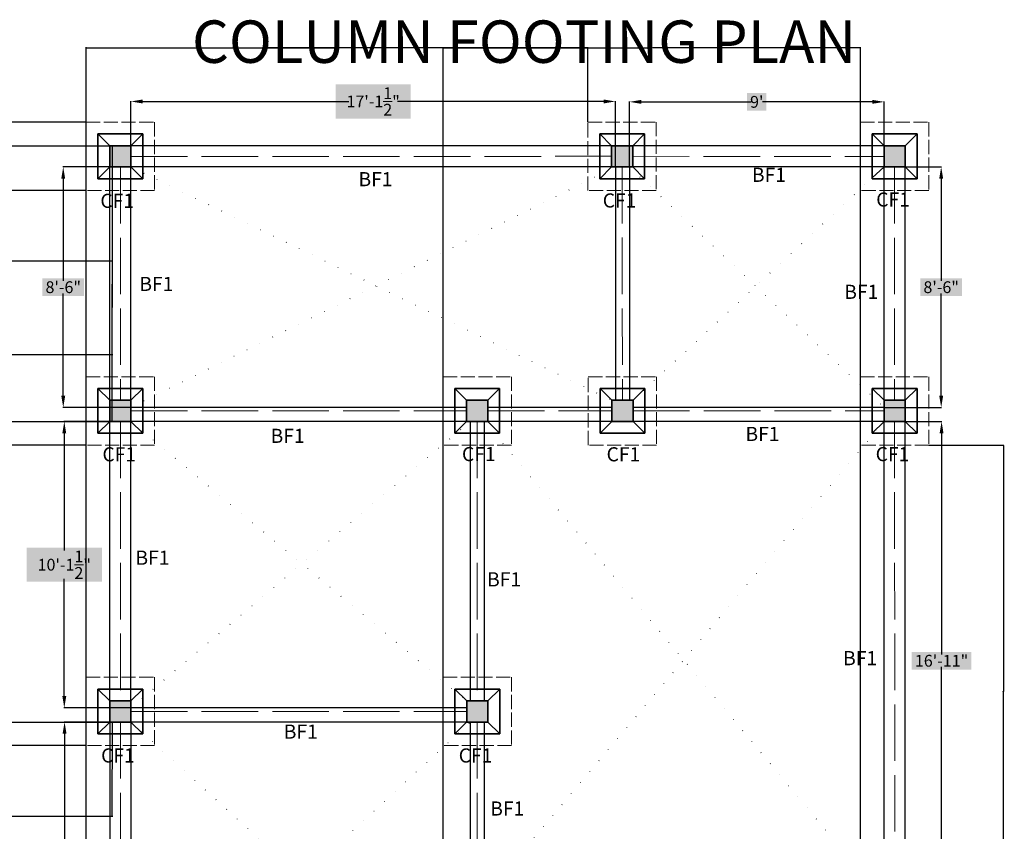
# Model space of a CAD drawing. Units: inches. Extents: x -301 to 715, y -607 to 364.
# Tile 141 of 141: x 194 to 612, y 19 to 364. Entities that reach past the tile are written whole.
import ezdxf

# ---------------------------------------------------------------- set-up
doc = ezdxf.new("R2010")
doc.units = ezdxf.units.IN
doc.header["$MEASUREMENT"] = 0
doc.linetypes.add('ACAD_ISO02W100', pattern=[15, 12, -3])
doc.linetypes.add('ACAD_ISO07W100', pattern=[3, 0, -3])
for name, color, linetype, lineweight in [('A-ANNO-DIMS', 2, 'Continuous', 18), ('A-ANNO-TITL', 1, 'Continuous', 35), ('S-ANNO-DIMS', 2, 'Continuous', 18), ('S-ANNO-TEXT', 240, 'Continuous', 18), ('S-BEAM-CNTR', 2, 'ACAD_ISO02W100', 13), ('S-COLS', 2, 'Continuous', 35), ('S-FNDN', 2, 'Continuous', 35), ('S-FNDN-HIDN', 220, 'ACAD_ISO02W100', 18)]:
    doc.layers.add(name, color=color, linetype=linetype, lineweight=lineweight)
for name, color, linetype, lineweight, true_color in [('S-BEAM', 152, 'Continuous', 30, 0x2776bb), ('S-COLS-PATT', 7, 'Continuous', 13, 0xffffff), ('S-FNDN-DIAG', 252, 'ACAD_ISO07W100', 13, 0x939598)]:
    doc.layers.add(name, color=color, linetype=linetype, lineweight=lineweight, true_color=true_color)
doc.styles.get("Standard").update_dxf_attribs({"font": 'arial.ttf'})
doc.dimstyles.get("Standard").update_dxf_attribs({"dimtxt": 0.18, "dimasz": 0.18, "dimexe": 0.18, "dimexo": 0.0625, "dimgap": 0.09, "dimtad": 0, "dimtih": 1, "dimtoh": 1, "dimdec": 1, "dimzin": 0, "dimdsep": 46, "dimlunit": 4, "dimtxsty": 'Standard', "dimcen": 0.09, "dimclrd": 3, "dimclre": 4, "dimclrt": 6, "dimadec": 0, "dimazin": 0, "dimtfac": 1, "dimtdec": 1, "dimtofl": 0, "dimtmove": 0, "dimatfit": 3, "dimfxl": 1, "dimtfill": 2, "dimtfillclr": 51, "dimtolj": 1, "dimtzin": 0, "dimarcsym": 0})

# ---------------------------------------------------------------- blocks, each defined once
blk = doc.blocks.new('*D63')
at = {"layer": 'Defpoints', "color": 0, "transparency": 16777216}
for p in [(560.89, 193.18), (585.29, 193.18), (560.89, -9.82)]:
    blk.add_point(p, dxfattribs=at)
at = {"layer": 'S-ANNO-DIMS', "color": 0, "lineweight": -2, "transparency": 16777216}
for p, q in [((560.95, 193.18), (585.47, 193.18)), ((585.29, 188.18), (585.29, 94.33)), ((585.29, -4.82), (585.29, 89.04)), ((560.95, -9.82), (585.47, -9.82))]:
    blk.add_line(p, q, dxfattribs=at)
at = {"layer": 'S-ANNO-DIMS', "color": 0, "transparency": 16777216}
for points in [[(584.46, 188.18), (586.12, 188.18), (585.29, 193.18)], [(584.46, -4.82), (586.12, -4.82), (585.29, -9.82)]]:
    blk.add_solid(points, dxfattribs=at)
at = {"layer": 'S-ANNO-DIMS', "color": 0, "transparency": 16777216, "insert": (585.29, 91.68), "char_height": 5, "attachment_point": 5, "bg_fill": 1, "box_fill_scale": 1.25, "bg_fill_color": 51, "bg_fill_transparency": 0}
blk.add_mtext('\\A1;16\'-11"', dxfattribs=at)
blk = doc.blocks.new('*D64')
at = {"layer": 'Defpoints', "color": 0, "transparency": 16777216}
for p in [(560.89, 301.18), (560.89, 199.18), (585.13, 199.18)]:
    blk.add_point(p, dxfattribs=at)
at = {"layer": 'S-ANNO-DIMS', "color": 0, "lineweight": -2, "transparency": 16777216}
for p, q in [((560.95, 301.18), (585.31, 301.18)), ((585.13, 296.18), (585.13, 252.83)), ((585.13, 204.18), (585.13, 247.54)), ((560.95, 199.18), (585.31, 199.18))]:
    blk.add_line(p, q, dxfattribs=at)
at = {"layer": 'S-ANNO-DIMS', "color": 0, "transparency": 16777216}
for points in [[(584.3, 296.18), (585.97, 296.18), (585.13, 301.18)], [(584.3, 204.18), (585.97, 204.18), (585.13, 199.18)]]:
    blk.add_solid(points, dxfattribs=at)
at = {"layer": 'S-ANNO-DIMS', "color": 0, "transparency": 16777216, "insert": (585.13, 250.18), "char_height": 5, "attachment_point": 5, "bg_fill": 1, "box_fill_scale": 1.25, "bg_fill_color": 51, "bg_fill_transparency": 0}
blk.add_mtext('\\A1;8\'-6"', dxfattribs=at)
blk = doc.blocks.new('*D65')
at = {"layer": 'Defpoints', "color": 0, "transparency": 16777216}
for p in [(560.89, 328.81), (452.89, 301.18), (560.89, 301.18)]:
    blk.add_point(p, dxfattribs=at)
at = {"layer": 'S-ANNO-DIMS', "color": 0, "lineweight": -2, "transparency": 16777216}
for p, q in [((452.89, 301.24), (452.89, 328.99)), ((457.89, 328.81), (504.5, 328.81)), ((555.89, 328.81), (509.28, 328.81)), ((560.89, 301.24), (560.89, 328.99))]:
    blk.add_line(p, q, dxfattribs=at)
at = {"layer": 'S-ANNO-DIMS', "color": 0, "transparency": 16777216}
for points in [[(457.89, 329.65), (457.89, 327.98), (452.89, 328.81)], [(555.89, 329.65), (555.89, 327.98), (560.89, 328.81)]]:
    blk.add_solid(points, dxfattribs=at)
at = {"layer": 'S-ANNO-DIMS', "color": 0, "transparency": 16777216, "insert": (506.89, 328.81), "char_height": 5, "attachment_point": 5, "bg_fill": 1, "box_fill_scale": 1.25, "bg_fill_color": 51, "bg_fill_transparency": 0}
blk.add_mtext("\\A1;9'", dxfattribs=at)
blk = doc.blocks.new('*D66')
at = {"layer": 'Defpoints', "color": 0, "transparency": 16777216}
for p in [(446.89, 328.98), (241.39, 301.18), (446.89, 300.92)]:
    blk.add_point(p, dxfattribs=at)
at = {"layer": 'S-ANNO-DIMS', "color": 0, "lineweight": -2, "transparency": 16777216}
for p, q in [((241.39, 301.24), (241.39, 329.16)), ((246.39, 328.98), (333.87, 328.98)), ((441.89, 328.98), (354.41, 328.98)), ((446.89, 300.99), (446.89, 329.16))]:
    blk.add_line(p, q, dxfattribs=at)
at = {"layer": 'S-ANNO-DIMS', "color": 0, "transparency": 16777216}
for points in [[(246.39, 329.81), (246.39, 328.14), (241.39, 328.98)], [(441.89, 329.81), (441.89, 328.14), (446.89, 328.98)]]:
    blk.add_solid(points, dxfattribs=at)
at = {"layer": 'S-ANNO-DIMS', "color": 0, "transparency": 16777216, "insert": (344.14, 328.98), "char_height": 5, "attachment_point": 5, "bg_fill": 1, "box_fill_scale": 1.25, "bg_fill_color": 51, "bg_fill_transparency": 0}
blk.add_mtext('\\A1;17\'-1{\\H1x;\\S1/2;}"', dxfattribs=at)
blk = doc.blocks.new('*D67')
at = {"layer": 'Defpoints', "color": 0, "transparency": 16777216}
for p in [(241.39, 301.18), (212.67, 199.18), (241.39, 199.18)]:
    blk.add_point(p, dxfattribs=at)
at = {"layer": 'S-ANNO-DIMS', "color": 0, "lineweight": -2, "transparency": 16777216}
for p, q in [((241.33, 301.18), (212.49, 301.18)), ((212.67, 296.18), (212.67, 252.83)), ((212.67, 204.18), (212.67, 247.54)), ((241.33, 199.18), (212.49, 199.18))]:
    blk.add_line(p, q, dxfattribs=at)
at = {"layer": 'S-ANNO-DIMS', "color": 0, "transparency": 16777216}
for points in [[(211.83, 296.18), (213.5, 296.18), (212.67, 301.18)], [(211.83, 204.18), (213.5, 204.18), (212.67, 199.18)]]:
    blk.add_solid(points, dxfattribs=at)
at = {"layer": 'S-ANNO-DIMS', "color": 0, "transparency": 16777216, "insert": (212.67, 250.18), "char_height": 5, "attachment_point": 5, "bg_fill": 1, "box_fill_scale": 1.25, "bg_fill_color": 51, "bg_fill_transparency": 0}
blk.add_mtext('\\A1;8\'-6"', dxfattribs=at)
blk = doc.blocks.new('*D68')
at = {"layer": 'Defpoints', "color": 0, "transparency": 16777216}
for p in [(241.39, 193.18), (213.11, 71.68), (241.39, 71.68)]:
    blk.add_point(p, dxfattribs=at)
at = {"layer": 'S-ANNO-DIMS', "color": 0, "lineweight": -2, "transparency": 16777216}
for p, q in [((241.33, 193.18), (212.93, 193.18)), ((213.11, 188.18), (213.11, 138.42)), ((213.11, 76.68), (213.11, 126.45)), ((241.33, 71.68), (212.93, 71.68))]:
    blk.add_line(p, q, dxfattribs=at)
at = {"layer": 'S-ANNO-DIMS', "color": 0, "transparency": 16777216}
for points in [[(212.28, 188.18), (213.94, 188.18), (213.11, 193.18)], [(212.28, 76.68), (213.94, 76.68), (213.11, 71.68)]]:
    blk.add_solid(points, dxfattribs=at)
at = {"layer": 'S-ANNO-DIMS', "color": 0, "transparency": 16777216, "insert": (213.11, 132.43), "char_height": 5, "attachment_point": 5, "bg_fill": 1, "box_fill_scale": 1.25, "bg_fill_color": 51, "bg_fill_transparency": 0}
blk.add_mtext('\\A1;10\'-1{\\H1x;\\S1/2;}"', dxfattribs=at)
blk = doc.blocks.new('*D69')
at = {"layer": 'Defpoints', "color": 0, "transparency": 16777216}
for p in [(241.39, 65.68), (213.23, -67.32), (241.39, -67.32)]:
    blk.add_point(p, dxfattribs=at)
at = {"layer": 'S-ANNO-DIMS', "color": 0, "lineweight": -2, "transparency": 16777216}
for p, q in [((241.33, 65.68), (213.05, 65.68)), ((213.23, 60.68), (213.23, 1.78)), ((213.23, -62.32), (213.23, -3.42)), ((241.33, -67.32), (213.05, -67.32))]:
    blk.add_line(p, q, dxfattribs=at)
at = {"layer": 'S-ANNO-DIMS', "color": 0, "transparency": 16777216}
for points in [[(212.4, 60.68), (214.06, 60.68), (213.23, 65.68)], [(212.4, -62.32), (214.06, -62.32), (213.23, -67.32)]]:
    blk.add_solid(points, dxfattribs=at)
at = {"layer": 'S-ANNO-DIMS', "color": 0, "transparency": 16777216, "insert": (213.23, -0.82), "char_height": 5, "attachment_point": 5, "bg_fill": 1, "box_fill_scale": 1.25, "bg_fill_color": 51, "bg_fill_transparency": 0}
blk.add_mtext('\\A1;11\'-1"', dxfattribs=at)
blk = doc.blocks.new('CF1-BASE-29')
at = {"ltscale": 0.5}
for p, q in [((0, 0), (0, 29)), ((0, 29), (29, 29)), ((29, 29), (29, 0)), ((29, 0), (0, 0))]:
    blk.add_line(p, q, dxfattribs=at)
blk = doc.blocks.new('CF1-SLOPED-PAD')
for p, q in [((0, 0), (0, 19)), ((0, 19), (19, 19)), ((0, 19), (5, 14)), ((14, 14), (19, 19)), ((19, 19), (19, 0)), ((0, 0), (5, 5)), ((14, 5), (19, 0)), ((19, 0), (0, 0))]:
    blk.add_line(p, q)
blk = doc.blocks.new('*D149')
at = {"layer": 'A-ANNO-DIMS', "color": 4, "lineweight": -2, "transparency": 16777216}
for p, q in [((-51.54, 65.68), (233.66, 65.68)), ((-51.54, 25.68), (233.66, 25.68))]:
    blk.add_line(p, q, dxfattribs=at)
at = {"layer": 'A-ANNO-DIMS', "color": 3, "lineweight": -2, "transparency": 16777216}
for p, q in [((233.48, 65.5), (233.48, 45.86)), ((233.48, 25.86), (233.48, 45.5))]:
    blk.add_line(p, q, dxfattribs=at)
at = {"layer": 'A-ANNO-DIMS', "color": 3, "transparency": 16777216}
for points in [[(233.45, 65.5), (233.51, 65.5), (233.48, 65.68)], [(233.45, 25.86), (233.51, 25.86), (233.48, 25.68)]]:
    blk.add_solid(points, dxfattribs=at)
at = {"layer": 'Defpoints', "color": 0, "transparency": 16777216}
for p in [(-51.6, 65.68), (-51.6, 25.68), (233.48, 25.68)]:
    blk.add_point(p, dxfattribs=at)
at = {"layer": 'A-ANNO-DIMS', "color": 6, "transparency": 16777216, "insert": (233.48, 45.68), "char_height": 0.18, "attachment_point": 5, "bg_fill": 1, "box_fill_scale": 1.25, "bg_fill_color": 51, "bg_fill_transparency": 0}
blk.add_mtext('\\A1;3\'-4"', dxfattribs=at)
blk = doc.blocks.new('*D153')
at = {"layer": 'A-ANNO-DIMS', "color": 4, "lineweight": -2, "transparency": 16777216}
for p, q in [((132.96, 310.18), (233.66, 310.18)), ((123.96, 193.18), (233.66, 193.18))]:
    blk.add_line(p, q, dxfattribs=at)
at = {"layer": 'A-ANNO-DIMS', "color": 3, "lineweight": -2, "transparency": 16777216}
for p, q in [((233.48, 310), (233.48, 251.86)), ((233.48, 193.36), (233.48, 251.5))]:
    blk.add_line(p, q, dxfattribs=at)
at = {"layer": 'A-ANNO-DIMS', "color": 3, "transparency": 16777216}
for points in [[(233.45, 310), (233.51, 310), (233.48, 310.18)], [(233.45, 193.36), (233.51, 193.36), (233.48, 193.18)]]:
    blk.add_solid(points, dxfattribs=at)
at = {"layer": 'Defpoints', "color": 0, "transparency": 16777216}
for p in [(132.9, 310.18), (123.9, 193.18), (233.48, 193.18)]:
    blk.add_point(p, dxfattribs=at)
at = {"layer": 'A-ANNO-DIMS', "color": 6, "transparency": 16777216, "insert": (233.48, 251.68), "char_height": 0.18, "attachment_point": 5, "bg_fill": 1, "box_fill_scale": 1.25, "bg_fill_color": 51, "bg_fill_transparency": 0}
blk.add_mtext('\\A1;9\'-9"', dxfattribs=at)
blk = doc.blocks.new('*D157')
at = {"layer": 'A-ANNO-DIMS', "color": 4, "lineweight": -2, "transparency": 16777216}
for p, q in [((-50.54, 261.43), (233.66, 261.43)), ((-50.54, 221.68), (233.66, 221.68))]:
    blk.add_line(p, q, dxfattribs=at)
at = {"layer": 'A-ANNO-DIMS', "color": 3, "lineweight": -2, "transparency": 16777216}
for p, q in [((233.48, 261.25), (233.48, 241.74)), ((233.48, 221.86), (233.48, 241.38))]:
    blk.add_line(p, q, dxfattribs=at)
at = {"layer": 'A-ANNO-DIMS', "color": 3, "transparency": 16777216}
for points in [[(233.45, 261.25), (233.51, 261.25), (233.48, 261.43)], [(233.45, 221.86), (233.51, 221.86), (233.48, 221.68)]]:
    blk.add_solid(points, dxfattribs=at)
at = {"layer": 'Defpoints', "color": 0, "transparency": 16777216}
for p in [(-50.6, 261.43), (233.48, 261.43), (-50.6, 221.68)]:
    blk.add_point(p, dxfattribs=at)
at = {"layer": 'A-ANNO-DIMS', "color": 6, "transparency": 16777216, "insert": (233.48, 241.56), "char_height": 0.18, "attachment_point": 5, "bg_fill": 1, "box_fill_scale": 1.25, "bg_fill_color": 51, "bg_fill_transparency": 0}
blk.add_mtext('\\A1;3\'-4"', dxfattribs=at)
blk = doc.blocks.new('*D162')
at = {"layer": 'A-ANNO-DIMS', "color": 4, "lineweight": -2, "transparency": 16777216}
for p, q in [((222.33, 320.18), (161.44, 320.18)), ((222.33, -233.82), (161.44, -233.82))]:
    blk.add_line(p, q, dxfattribs=at)
at = {"layer": 'A-ANNO-DIMS', "color": 3, "lineweight": -2, "transparency": 16777216}
for p, q in [((161.62, 320), (161.62, 43.36)), ((161.62, -233.64), (161.62, 43))]:
    blk.add_line(p, q, dxfattribs=at)
at = {"layer": 'A-ANNO-DIMS', "color": 3, "transparency": 16777216}
for points in [[(161.59, 320), (161.65, 320), (161.62, 320.18)], [(161.59, -233.64), (161.65, -233.64), (161.62, -233.82)]]:
    blk.add_solid(points, dxfattribs=at)
at = {"layer": 'Defpoints', "color": 0, "transparency": 16777216}
for p in [(161.62, 320.18), (222.39, 320.18), (222.39, -233.82)]:
    blk.add_point(p, dxfattribs=at)
at = {"layer": 'A-ANNO-DIMS', "color": 6, "transparency": 16777216, "insert": (161.62, 43.18), "char_height": 0.18, "attachment_point": 5, "bg_fill": 1, "box_fill_scale": 1.25, "bg_fill_color": 51, "bg_fill_transparency": 0}
blk.add_mtext('\\A1;46\'-2"', dxfattribs=at)
blk = doc.blocks.new('*D163')
at = {"layer": 'A-ANNO-DIMS', "color": 4, "lineweight": -2, "transparency": 16777216}
for p, q in [((222.39, -204.76), (222.39, 351.98)), ((373.83, -204.75), (373.83, 351.98))]:
    blk.add_line(p, q, dxfattribs=at)
at = {"layer": 'A-ANNO-DIMS', "color": 3, "lineweight": -2, "transparency": 16777216}
for p, q in [((222.57, 351.8), (297.51, 351.8)), ((373.65, 351.8), (298.71, 351.8))]:
    blk.add_line(p, q, dxfattribs=at)
at = {"layer": 'A-ANNO-DIMS', "color": 3, "transparency": 16777216}
for points in [[(222.57, 351.83), (222.57, 351.77), (222.39, 351.8)], [(373.65, 351.83), (373.65, 351.77), (373.83, 351.8)]]:
    blk.add_solid(points, dxfattribs=at)
at = {"layer": 'Defpoints', "color": 0, "transparency": 16777216}
for p in [(373.83, 351.8), (222.39, -204.82), (373.83, -204.81)]:
    blk.add_point(p, dxfattribs=at)
at = {"layer": 'A-ANNO-DIMS', "color": 6, "transparency": 16777216, "insert": (298.11, 351.8), "char_height": 0.18, "attachment_point": 5, "bg_fill": 1, "box_fill_scale": 1.25, "bg_fill_color": 51, "bg_fill_transparency": 0}
blk.add_mtext('\\A1;12\'-7 1/2"', dxfattribs=at)
blk = doc.blocks.new('*D164')
at = {"layer": 'A-ANNO-DIMS', "color": 4, "lineweight": -2, "transparency": 16777216}
for p, q in [((373.83, -204.75), (373.83, 351.98)), ((550.9, -204.77), (550.9, 351.98))]:
    blk.add_line(p, q, dxfattribs=at)
at = {"layer": 'A-ANNO-DIMS', "color": 3, "lineweight": -2, "transparency": 16777216}
for p, q in [((374.01, 351.8), (461.97, 351.8)), ((550.72, 351.8), (462.76, 351.8))]:
    blk.add_line(p, q, dxfattribs=at)
at = {"layer": 'A-ANNO-DIMS', "color": 3, "transparency": 16777216}
for points in [[(374.01, 351.83), (374.01, 351.77), (373.83, 351.8)], [(550.72, 351.83), (550.72, 351.77), (550.9, 351.8)]]:
    blk.add_solid(points, dxfattribs=at)
at = {"layer": 'Defpoints', "color": 0, "transparency": 16777216}
for p in [(550.9, 351.8), (373.83, -204.81), (550.9, -204.83)]:
    blk.add_point(p, dxfattribs=at)
at = {"layer": 'A-ANNO-DIMS', "color": 6, "transparency": 16777216, "insert": (462.36, 351.8), "char_height": 0.18, "attachment_point": 5, "bg_fill": 1, "box_fill_scale": 1.25, "bg_fill_color": 51, "bg_fill_transparency": 0}
blk.add_mtext('\\A1;14\'-9"', dxfattribs=at)
blk = doc.blocks.new('*D165')
at = {"layer": 'A-ANNO-DIMS', "color": 4, "lineweight": -2, "transparency": 16777216}
for p, q in [((222.39, 320.24), (222.39, 351.98)), ((435.27, 320.26), (435.27, 351.98))]:
    blk.add_line(p, q, dxfattribs=at)
at = {"layer": 'A-ANNO-DIMS', "color": 3, "lineweight": -2, "transparency": 16777216}
for p, q in [((222.57, 351.8), (328.44, 351.8)), ((435.09, 351.8), (329.22, 351.8))]:
    blk.add_line(p, q, dxfattribs=at)
at = {"layer": 'A-ANNO-DIMS', "color": 3, "transparency": 16777216}
for points in [[(222.57, 351.83), (222.57, 351.77), (222.39, 351.8)], [(435.09, 351.83), (435.09, 351.77), (435.27, 351.8)]]:
    blk.add_solid(points, dxfattribs=at)
at = {"layer": 'Defpoints', "color": 0, "transparency": 16777216}
for p in [(435.27, 351.8), (222.39, 320.18), (435.27, 320.2)]:
    blk.add_point(p, dxfattribs=at)
at = {"layer": 'A-ANNO-DIMS', "color": 6, "transparency": 16777216, "insert": (328.83, 351.8), "char_height": 0.18, "attachment_point": 5, "bg_fill": 1, "box_fill_scale": 1.25, "bg_fill_color": 51, "bg_fill_transparency": 0}
blk.add_mtext('\\A1;17\'-9"', dxfattribs=at)
blk = doc.blocks.new('*D168')
at = {"layer": 'A-ANNO-DIMS', "color": 4, "lineweight": -2, "transparency": 16777216}
for p, q in [((222.33, 55.68), (161.44, 55.68)), ((222.33, -83.32), (161.44, -83.32))]:
    blk.add_line(p, q, dxfattribs=at)
at = {"layer": 'A-ANNO-DIMS', "color": 3, "lineweight": -2, "transparency": 16777216}
for p, q in [((161.62, 55.5), (161.62, -13.64)), ((161.62, -83.14), (161.62, -14))]:
    blk.add_line(p, q, dxfattribs=at)
at = {"layer": 'A-ANNO-DIMS', "color": 3, "transparency": 16777216}
for points in [[(161.59, 55.5), (161.65, 55.5), (161.62, 55.68)], [(161.59, -83.14), (161.65, -83.14), (161.62, -83.32)]]:
    blk.add_solid(points, dxfattribs=at)
at = {"layer": 'Defpoints', "color": 0, "transparency": 16777216}
for p in [(161.62, 55.68), (222.39, 55.68), (222.39, -83.32)]:
    blk.add_point(p, dxfattribs=at)
at = {"layer": 'A-ANNO-DIMS', "color": 6, "transparency": 16777216, "insert": (161.62, -13.82), "char_height": 0.18, "attachment_point": 5, "bg_fill": 1, "box_fill_scale": 1.25, "bg_fill_color": 51, "bg_fill_transparency": 0}
blk.add_mtext('\\A1;11\'-7"', dxfattribs=at)
blk = doc.blocks.new('*D169')
at = {"layer": 'A-ANNO-DIMS', "color": 4, "lineweight": -2, "transparency": 16777216}
for p, q in [((222.33, 183.18), (161.44, 183.18)), ((222.33, 55.68), (161.44, 55.68))]:
    blk.add_line(p, q, dxfattribs=at)
at = {"layer": 'A-ANNO-DIMS', "color": 3, "lineweight": -2, "transparency": 16777216}
for p, q in [((161.62, 183), (161.62, 119.62)), ((161.62, 55.86), (161.62, 119.25))]:
    blk.add_line(p, q, dxfattribs=at)
at = {"layer": 'A-ANNO-DIMS', "color": 3, "transparency": 16777216}
for points in [[(161.59, 183), (161.65, 183), (161.62, 183.18)], [(161.59, 55.86), (161.65, 55.86), (161.62, 55.68)]]:
    blk.add_solid(points, dxfattribs=at)
at = {"layer": 'Defpoints', "color": 0, "transparency": 16777216}
for p in [(161.62, 183.18), (222.39, 183.18), (222.39, 55.68)]:
    blk.add_point(p, dxfattribs=at)
at = {"layer": 'A-ANNO-DIMS', "color": 6, "transparency": 16777216, "insert": (161.62, 119.43), "char_height": 0.18, "attachment_point": 5, "bg_fill": 1, "box_fill_scale": 1.25, "bg_fill_color": 51, "bg_fill_transparency": 0}
blk.add_mtext('\\A1;10\'-7 1/2"', dxfattribs=at)
blk = doc.blocks.new('*D170')
at = {"layer": 'A-ANNO-DIMS', "color": 4, "lineweight": -2, "transparency": 16777216}
for p, q in [((222.33, 291.18), (161.44, 291.18)), ((222.33, 183.18), (161.44, 183.18))]:
    blk.add_line(p, q, dxfattribs=at)
at = {"layer": 'A-ANNO-DIMS', "color": 3, "lineweight": -2, "transparency": 16777216}
for p, q in [((161.62, 291), (161.62, 237.36)), ((161.62, 183.36), (161.62, 237))]:
    blk.add_line(p, q, dxfattribs=at)
at = {"layer": 'A-ANNO-DIMS', "color": 3, "transparency": 16777216}
for points in [[(161.59, 291), (161.65, 291), (161.62, 291.18)], [(161.59, 183.36), (161.65, 183.36), (161.62, 183.18)]]:
    blk.add_solid(points, dxfattribs=at)
at = {"layer": 'Defpoints', "color": 0, "transparency": 16777216}
for p in [(161.62, 291.18), (222.39, 291.18), (222.39, 183.18)]:
    blk.add_point(p, dxfattribs=at)
at = {"layer": 'A-ANNO-DIMS', "color": 6, "transparency": 16777216, "insert": (161.62, 237.18), "char_height": 0.18, "attachment_point": 5, "bg_fill": 1, "box_fill_scale": 1.25, "bg_fill_color": 51, "bg_fill_transparency": 0}
blk.add_mtext('\\A1;9\'-0"', dxfattribs=at)
blk = doc.blocks.new('*D174')
at = {"layer": 'A-ANNO-DIMS', "color": 4, "lineweight": -2, "transparency": 16777216}
for p, q in [((579.95, 183.18), (611.7, 183.18)), ((579.98, -25.82), (611.7, -25.82))]:
    blk.add_line(p, q, dxfattribs=at)
at = {"layer": 'A-ANNO-DIMS', "color": 3, "lineweight": -2, "transparency": 16777216}
for p, q in [((611.52, 183), (611.52, 78.86)), ((611.52, -25.64), (611.52, 78.5))]:
    blk.add_line(p, q, dxfattribs=at)
at = {"layer": 'A-ANNO-DIMS', "color": 3, "transparency": 16777216}
for points in [[(611.49, 183), (611.55, 183), (611.52, 183.18)], [(611.49, -25.64), (611.55, -25.64), (611.52, -25.82)]]:
    blk.add_solid(points, dxfattribs=at)
at = {"layer": 'Defpoints', "color": 0, "transparency": 16777216}
for p in [(579.89, 183.18), (611.52, 183.18), (579.92, -25.82)]:
    blk.add_point(p, dxfattribs=at)
at = {"layer": 'A-ANNO-DIMS', "color": 6, "transparency": 16777216, "insert": (611.52, 78.68), "char_height": 0.18, "attachment_point": 5, "bg_fill": 1, "box_fill_scale": 1.25, "bg_fill_color": 51, "bg_fill_transparency": 0}
blk.add_mtext('\\A1;17\'-5"', dxfattribs=at)

msp = doc.modelspace()

# ---------------------------------------------------------------- hatches: boundary and pattern name
at = {"layer": 'S-COLS-PATT'}
h = msp.add_hatch(color=256, dxfattribs=at)
h.dxf.hatch_style = 1
h.paths.add_polyline_path([(241.39, 310.18), (232.39, 310.18), (232.39, 301.18), (241.39, 301.18)])
h.paths.add_polyline_path([(445.27, 310.18), (445.27, 301.2), (454.27, 301.2), (454.27, 310.18)])
h.paths.add_polyline_path([(560.89, 310.18), (560.89, 301.18), (569.89, 301.18), (569.89, 310.18)])
h.paths.add_polyline_path([(241.39, 202.18), (232.39, 202.18), (232.39, 193.18), (241.39, 193.18)])
h.paths.add_polyline_path([(383.81, 202.18), (383.81, 193.18), (392.81, 193.18), (392.81, 202.18)])
h.paths.add_polyline_path([(445.41, 202.18), (445.41, 193.18), (454.41, 193.18), (454.41, 202.18)])
h.paths.add_polyline_path([(560.89, 202.18), (560.89, 193.18), (569.89, 193.18), (569.89, 202.18)])
h.paths.add_polyline_path([(241.39, 65.68), (241.39, 74.68), (232.39, 74.68), (232.39, 65.68)])
h.paths.add_polyline_path([(392.83, 65.66), (392.83, 74.66), (383.83, 74.66), (383.83, 65.66)])
h.paths.add_polyline_path([(560.92, -6.82), (560.92, -15.82), (569.89, -15.82), (569.89, -9.82), (569.89, -6.82)])
h.paths.add_polyline_path([(466.35, -15.82), (466.35, -6.82), (457.35, -6.82), (457.35, -15.82)])
h.paths.add_polyline_path([(383.83, -15.78), (392.83, -15.78), (392.83, -6.78), (383.83, -6.78)])
h.paths.add_polyline_path([(241.39, -64.32), (232.39, -64.32), (232.39, -73.32), (241.39, -73.32)])
h.paths.add_polyline_path([(392.85, -64.32), (383.85, -64.32), (383.85, -73.32), (392.85, -73.32)])
h.paths.add_polyline_path([(466.37, -73.82), (457.37, -73.82), (457.37, -82.82), (466.37, -82.82)])
h.paths.add_polyline_path([(560.89, -73.82), (560.89, -82.82), (569.89, -82.82), (569.89, -73.82)])
h.paths.add_polyline_path([(560.89, -121.82), (560.89, -130.82), (569.89, -130.82), (569.89, -121.82)])
h.paths.add_polyline_path([(569.89, -214.83), (560.9, -214.83), (560.9, -223.82), (569.89, -223.82)])
h.paths.add_polyline_path([(392.83, -223.81), (392.83, -214.82), (391.39, -214.82), (385.39, -214.81), (385.39, -214.82), (383.83, -214.82), (383.83, -223.81)])
h.paths.add_polyline_path([(392.83, -121.74), (383.83, -121.74), (383.83, -130.74), (392.83, -130.74)])
h.paths.add_polyline_path([(241.39, -223.82), (241.39, -214.82), (232.39, -214.82), (232.39, -223.82)])

# ---------------------------------------------------------------- linework, layer by layer
at = {"layer": 'S-BEAM'}
for p, q in [((232.39, 71.68), (232.39, 310.18)), ((569.89, 310.18), (232.39, 310.18)), ((569.89, 199.18), (569.89, 310.18)), ((241.39, 199.18), (241.39, 301.18)), ((446.89, 301.18), (241.39, 301.18)), ((446.89, 301.18), (446.89, 202.18)), ((560.89, 301.18), (452.89, 301.18)), ((452.89, 301.18), (452.89, 202.18)), ((560.89, 199.18), (560.89, 301.18)), ((241.39, 199.18), (241.39, 215.68)), ((383.81, 199.18), (241.39, 199.18)), ((445.41, 199.18), (392.81, 199.18)), ((560.89, 199.18), (454.41, 199.18)), ((569.89, -9.82), (569.89, 199.18)), ((241.39, 71.68), (241.39, 193.18)), ((383.81, 193.18), (241.39, 193.18)), ((385.39, 74.66), (385.39, 193.18)), ((391.39, 74.66), (391.39, 193.18)), ((452.89, 193.18), (392.81, 193.18)), ((560.89, 193.18), (452.89, 193.18)), ((560.89, -9.82), (560.89, 193.18)), ((232.39, 71.68), (232.39, -67.32)), ((383.83, 71.68), (241.39, 71.68)), ((383.81, 65.68), (241.39, 65.68)), ((241.39, 65.68), (241.39, -67.32)), ((385.39, -6.78), (385.39, 65.66)), ((391.39, -6.82), (391.39, 65.68))]:
    msp.add_line(p, q, dxfattribs=at)
at = {"layer": 'S-BEAM-CNTR', "ltscale": 2}
for p, q in [((241.39, 305.68), (445.27, 305.7)), ((454.27, 305.7), (560.89, 305.68)), ((236.89, 301.18), (236.89, 202.18)), ((449.77, 301.2), (449.9, 202.18)), ((565.39, 301.18), (565.39, 202.18)), ((241.39, 197.68), (383.81, 197.68)), ((392.81, 197.68), (445.41, 197.68)), ((454.41, 197.68), (560.89, 197.68)), ((236.89, 193.18), (236.89, 74.68)), ((388.31, 193.18), (388.33, 74.66)), ((565.39, 193.18), (565.4, -6.82)), ((241.39, 70.18), (383.83, 70.16)), ((236.89, 65.68), (236.89, -64.32)), ((388.33, 65.68), (388.33, -6.78))]:
    msp.add_line(p, q, dxfattribs=at)
at = {"layer": 'S-BEAM-CNTR'}
for p, q in [((385.39, 65.66), (385.39, 65.68)), ((391.39, 65.66), (391.39, 65.68))]:
    msp.add_line(p, q, dxfattribs=at)
at = {"layer": 'S-COLS'}
for p, q in [((232.39, 310.18), (241.39, 310.18)), ((232.39, 301.18), (232.39, 310.18)), ((241.39, 310.18), (241.39, 301.18)), ((445.27, 310.2), (454.27, 310.2)), ((445.27, 301.2), (445.27, 310.2)), ((454.27, 310.2), (454.27, 301.2)), ((560.89, 310.18), (569.89, 310.18)), ((560.89, 301.18), (560.89, 310.18)), ((569.89, 310.18), (569.89, 301.18)), ((241.39, 301.18), (232.39, 301.18)), ((454.27, 301.2), (445.27, 301.2)), ((569.89, 301.18), (560.89, 301.18)), ((232.39, 202.18), (241.39, 202.18)), ((232.39, 193.18), (232.39, 202.18)), ((241.39, 202.18), (241.39, 193.18)), ((383.81, 202.18), (392.81, 202.18)), ((383.81, 193.18), (383.81, 202.18)), ((392.81, 202.18), (392.81, 193.18)), ((445.41, 202.18), (454.41, 202.18)), ((445.41, 193.18), (445.41, 202.18)), ((454.41, 202.18), (454.41, 193.18)), ((560.89, 202.18), (569.89, 202.18)), ((560.89, 193.18), (560.89, 202.18)), ((569.89, 202.18), (569.89, 193.18)), ((241.39, 193.18), (232.39, 193.18)), ((392.81, 193.18), (383.81, 193.18)), ((454.41, 193.18), (445.41, 193.18)), ((569.89, 193.18), (560.89, 193.18)), ((232.39, 74.68), (241.39, 74.68)), ((232.39, 65.68), (232.39, 74.68)), ((241.39, 74.68), (241.39, 65.68)), ((383.83, 74.66), (392.83, 74.66)), ((383.83, 65.66), (383.83, 74.66)), ((392.83, 74.66), (392.83, 65.66)), ((241.39, 65.68), (232.39, 65.68)), ((392.83, 65.66), (383.83, 65.66))]:
    msp.add_line(p, q, dxfattribs=at)
at = {"layer": 'S-FNDN'}
for p, q in [((440.27, 315.2), (459.27, 315.2)), ((440.27, 296.2), (440.27, 315.2)), ((440.27, 315.2), (445.27, 310.2)), ((454.27, 310.18), (459.27, 315.2)), ((459.27, 315.2), (459.27, 296.2)), ((555.89, 296.18), (555.89, 315.18)), ((555.89, 315.18), (574.89, 315.18)), ((555.89, 315.18), (560.89, 310.18)), ((569.89, 310.18), (574.89, 315.18)), ((574.89, 315.18), (574.89, 296.18)), ((440.27, 296.2), (445.27, 301.2)), ((454.27, 301.2), (459.27, 296.2)), ((555.89, 296.53), (560.89, 301.18)), ((569.89, 301.18), (574.89, 296.18)), ((459.27, 296.2), (440.27, 296.2)), ((574.89, 296.18), (555.89, 296.18)), ((378.83, 60.66), (378.83, 79.66)), ((378.83, 79.66), (397.83, 79.66)), ((378.83, 79.66), (383.83, 74.66)), ((392.83, 74.66), (397.83, 79.66)), ((397.83, 79.66), (397.83, 60.66)), ((378.83, 60.66), (383.81, 65.68)), ((392.83, 65.66), (397.83, 60.66)), ((397.83, 60.66), (378.83, 60.66))]:
    msp.add_line(p, q, dxfattribs=at)
at = {"layer": 'S-FNDN-DIAG', "ltscale": 2}
for p, q in [((241.39, 199.18), (446.89, 301.18)), ((241.39, 301.18), (445.41, 202.18)), ((452.89, 301.18), (560.89, 199.18)), ((454.41, 202.18), (560.89, 301.18)), ((241.39, 71.68), (385.39, 193.18)), ((241.39, 193.18), (383.83, 74.66)), ((391.39, 193.18), (560.89, -9.82)), ((392.83, -6.78), (560.89, 193.18)), ((241.39, 65.68), (383.85, -64.32)), ((241.39, -67.32), (385.39, 65.66))]:
    msp.add_line(p, q, dxfattribs=at)

# ---------------------------------------------------------------- block references
at = {"layer": 'S-FNDN'}
for p, rotation in [((246.39, 296.18), 89.9999999999993), ((397.81, 207.18), 180), ((459.41, 207.18), 180), ((555.89, 207.18), 270.0000000000001), ((246.39, 60.68), 89.99999999999969)]:
    msp.add_blockref('CF1-SLOPED-PAD', p, dxfattribs=dict(at, rotation=rotation))
msp.add_blockref('CF1-SLOPED-PAD', (227.39, 188.18), dxfattribs=at)
at = {"layer": 'S-FNDN-HIDN'}
for p, rotation in [((222.39, 320.18), 270), ((464.27, 320.2), 180), ((579.89, 291.18), 89.99999999999976), ((251.39, 212.18), 180), ((579.89, 183.18), 89.99999999999976), ((222.39, 84.68), 270), ((402.83, 55.66), 90)]:
    msp.add_blockref('CF1-BASE-29', p, dxfattribs=dict(at, rotation=rotation))
for p in [(373.81, 183.18), (435.41, 183.18)]:
    msp.add_blockref('CF1-BASE-29', p, dxfattribs=at)

# ---------------------------------------------------------------- texts
at = {"layer": 'A-ANNO-TITL'}
msp.add_text('COLUMN FOOTING PLAN', height=18, dxfattribs=at).set_placement((267.3, 345.35))
at = {"layer": 'S-ANNO-TEXT'}
for s, p in [('BF1', (504.83, 294.87)), ('BF1', (337.91, 293.01)), ('CF1', (228.41, 283.82)), ('CF1', (441.54, 283.97)), ('CF1', (557.57, 284.37)), ('BF1', (244.96, 248.57)), ('BF1', (544, 245.21)), ('BF1', (300.63, 184.11)), ('BF1', (502.09, 184.92)), ('CF1', (229.28, 176.28)), ('CF1', (381.81, 176.37)), ('CF1', (443.17, 176.29)), ('CF1', (557.32, 176.35)), ('BF1', (243.29, 132.4)), ('BF1', (392.48, 123.22)), ('BF1', (543.52, 89.79)), ('BF1', (306.22, 58.62)), ('CF1', (228.72, 48.5)), ('CF1', (380.44, 48.49)), ('BF1', (393.81, 25.99))]:
    msp.add_text(s, height=6, dxfattribs=at).set_placement(p)

# ---------------------------------------------------------------- dimensions: what is measured, and where the dimension line sits
at = {"layer": 'A-ANNO-DIMS'}
for base, p1, p2, picture, middle in [((373.83, 351.8), (222.39, -204.82), (373.83, -204.81), '*D163', (298.11, 351.8)), ((435.27, 351.8), (222.39, 320.18), (435.27, 320.2), '*D165', (328.83, 351.8)), ((550.9, 351.8), (373.83, -204.81), (550.9, -204.83), '*D164', (462.36, 351.8))]:
    dim = msp.add_linear_dim(base=base, p1=p1, p2=p2, dimstyle='Standard', override={"dimdec": 1, "dimlfac": 1, "dimrnd": 0, "dimzin": 1, "dimdsep": 46, "dimlunit": 4, "dimfrac": 2}, dxfattribs=at)
    dim.commit()
    dim.dimension.update_dxf_attribs({"geometry": picture, "text_midpoint": middle})
for base, p1, p2, picture, middle in [((161.62, 320.18), (222.39, -233.82), (222.39, 320.18), '*D162', (161.62, 43.18)), ((233.48, 193.18), (132.9, 310.18), (123.9, 193.18), '*D153', (233.48, 251.68)), ((161.62, 291.18), (222.39, 183.18), (222.39, 291.18), '*D170', (161.62, 237.18)), ((233.479242, 261.43233), (-50.603288, 221.68233), (-50.603288, 261.43233), '*D157', (233.479242, 241.55733)), ((161.62, 183.18), (222.39, 55.68), (222.39, 183.18), '*D169', (161.62, 119.43)), ((611.52, 183.18), (579.92, -25.82), (579.89, 183.18), '*D174', (611.52, 78.68)), ((233.48, 25.68), (-51.6, 65.68), (-51.6, 25.68), '*D149', (233.48, 45.68)), ((161.62, 55.68), (222.39, -83.32), (222.39, 55.68), '*D168', (161.62, -13.82))]:
    dim = msp.add_linear_dim(base=base, p1=p1, p2=p2, angle=90, dimstyle='Standard', override={"dimdec": 1, "dimlfac": 1, "dimrnd": 0, "dimzin": 1, "dimdsep": 46, "dimlunit": 4, "dimfrac": 2}, dxfattribs=at)
    dim.commit()
    dim.dimension.update_dxf_attribs({"geometry": picture, "text_midpoint": middle})
at = {"layer": 'S-ANNO-DIMS'}
for base, p1, p2, picture, middle in [((446.89, 328.98), (241.39, 301.18), (446.89, 300.92), '*D66', (344.14, 328.98)), ((560.89, 328.81), (452.89, 301.18), (560.89, 301.18), '*D65', (506.89, 328.81))]:
    dim = msp.add_linear_dim(base=base, p1=p1, p2=p2, dimstyle='Standard', override={"dimtxt": 5, "dimasz": 5, "dimclrd": 0, "dimclre": 0, "dimclrt": 0}, dxfattribs=at)
    dim.commit()
    dim.dimension.update_dxf_attribs({"geometry": picture, "text_midpoint": middle})
for base, p1, p2, picture, middle in [((212.67, 199.18), (241.39, 301.18), (241.39, 199.18), '*D67', (212.67, 250.18)), ((585.13, 199.18), (560.89, 301.18), (560.89, 199.18), '*D64', (585.13, 250.18)), ((213.11, 71.68), (241.39, 193.18), (241.39, 71.68), '*D68', (213.11, 132.43)), ((585.29, 193.18), (560.89, -9.82), (560.89, 193.18), '*D63', (585.29, 91.68)), ((213.23, -67.32), (241.39, 65.68), (241.39, -67.32), '*D69', (213.23, -0.82))]:
    dim = msp.add_linear_dim(base=base, p1=p1, p2=p2, angle=90, dimstyle='Standard', override={"dimtxt": 5, "dimasz": 5, "dimclrd": 0, "dimclre": 0, "dimclrt": 0}, dxfattribs=at)
    dim.commit()
    dim.dimension.update_dxf_attribs({"geometry": picture, "text_midpoint": middle})

doc.saveas('drawing.dxf')
